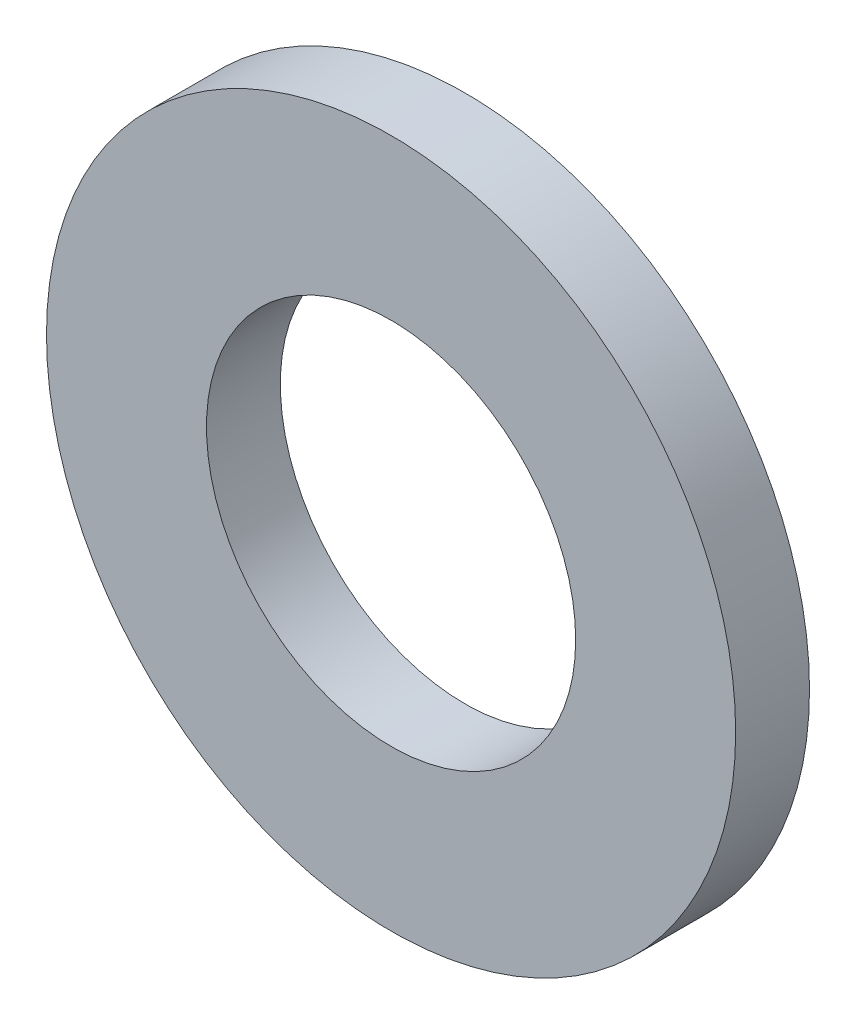
from build123d import *

# Parameters (mm, degrees)
WASHER_PROFILE_28_15_R   = 14
WASHER_PROFILE_28_15_R_2 = 7.5
WASHER_BODY_3MM_DEPTH    = 1.5


with BuildPart() as part:
    # Washer Profile Ø28-Ø15 → Washer Body 3mm (new, symmetric)
    with BuildSketch(Plane.XY):
        Circle(WASHER_PROFILE_28_15_R)
        Circle(WASHER_PROFILE_28_15_R_2, mode=Mode.SUBTRACT)
    extrude(amount=WASHER_BODY_3MM_DEPTH, both=True)


solid = part.part
